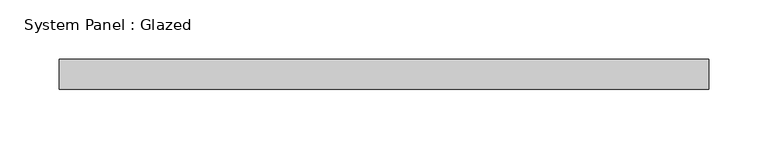
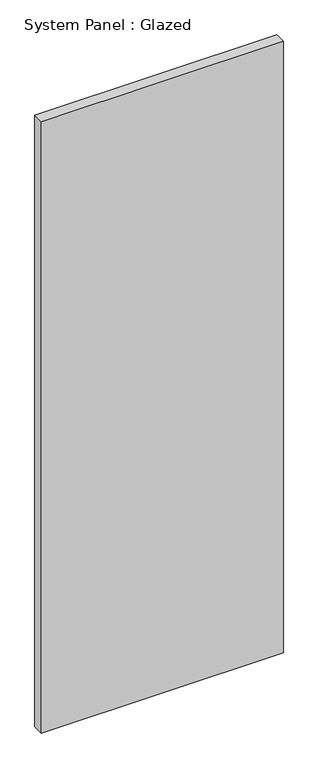
"""IFC4 building model written with IfcOpenShell, lengths in millimetres: plate geometry, System Panel : Glazed."""

from ifc_helpers import new_model, si_unit, origin, origin_with_axes, place, context, project, spatial, polyline, outline, extrude, source, transform, mapped, element, save


def system_panel_glazed_9988b647(model_context):
    return source(origin(), model_context, "Body", "SweptSolid", [
        extrude(outline(polyline([(274.1083333, 19.05), (-274.1083333, 19.05), (-274.1083333, 44.45), (274.1083333, 44.45), (274.1083333, 19.05)])), origin_with_axes(), (0.0, 0.0, 1.0), 1463.48195),
    ])


if __name__ == "__main__":
    model = new_model("IFC4")
    model_context = context("Model", 3, world=origin())
    ifc_project = project(units=[si_unit("LENGTHUNIT", "METRE", prefix="MILLI")], contexts=[model_context])
    site = spatial("IfcSite", under=ifc_project)
    building = spatial("IfcBuilding", under=site)
    placement = place(None, origin())
    system_panel_glazed_shape = system_panel_glazed_9988b647(model_context)
    element("IfcPlate", 1, ObjectType="System Panel : Glazed", at=placement, inside=building, context=model_context, shape_type="MappedRepresentation", body=[
        mapped(system_panel_glazed_shape, transform((0.0, 0.0, 0.0), x_axis=(1.0, 0.0, 0.0), y_axis=(0.0, 1.0, 0.0), z_axis=(0.0, 0.0, 1.0))),
    ])
    save(model, "model.ifc")

# Revit data of these elements
# Type "System Panel : Glazed"
#   Construction Type Id = "GSP4R"
#   Analytic Construction = "1/8 in Pilkington single glazing"
#   Visual Light Transmittance = 0.9
#   Solar Heat Gain Coefficient = 0.86
#   Heat Transfer Coefficient (U) = 1.18115 BTU/(h·ft²·°F)
# Element 1 (IfcPlate, "System Panel : Glazed")
#   Materials on its faces: "Glass"
# Materials
#   "Glass": class "Glass", colour RGB 0 128 192, transparency 0.75, Description = "Soda Lime Glass", Cost = 0
